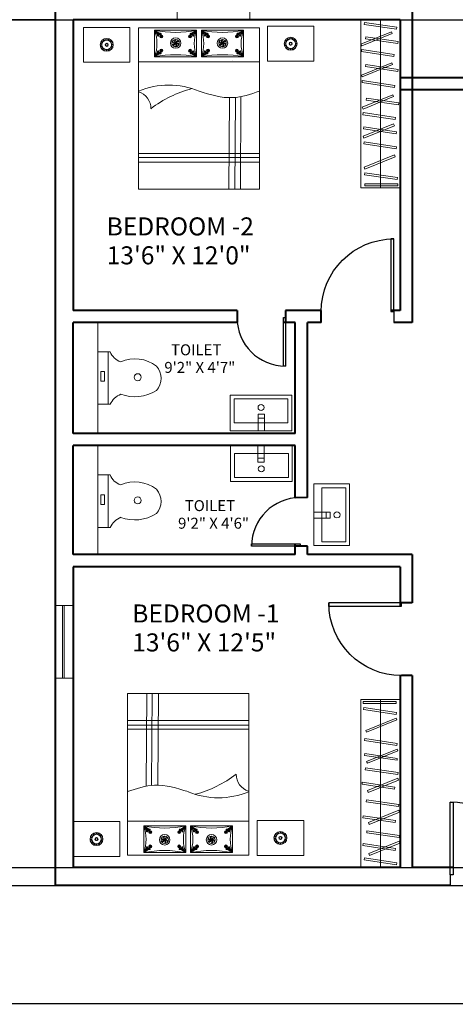
# Model space of a CAD drawing. Units: inches. Extents: x -46 to 1145, y -527 to 760.
# Tile 17 of 57: x 573 to 788, y -527 to -39. Entities that reach past the tile are written whole.
import ezdxf

# ---------------------------------------------------------------- set-up
doc = ezdxf.new("R2010")
doc.units = ezdxf.units.IN
doc.header["$MEASUREMENT"] = 0
for name, color, linetype, lineweight in [('A-ANNO-DIMS', 2, 'Continuous', 18), ('A-AREA-IDEN', 1, 'Continuous', 18), ('A-FLOR-CASE', 32, 'Continuous', 18), ('A-FLOR-FIXT', 9, 'Continuous', 18), ('A-FURN', 2, 'Continuous', 13), ('C-SITE', 7, 'Continuous', 30), ('DOORS', 3, 'Continuous', 25), ('WALLS', 4, 'Continuous', 40), ('WINDOWS', 240, 'Continuous', 20)]:
    doc.layers.add(name, color=color, linetype=linetype, lineweight=lineweight)
doc.layers.add('FURNTIURE', color=2, linetype='Continuous')
doc.layers.add('LT', color=9, linetype='Continuous')
doc.styles.get("Standard").update_dxf_attribs({"font": 'arial.ttf'})
doc.dimstyles.get("Standard").update_dxf_attribs({"dimtxt": 0.18, "dimasz": 0.18, "dimexe": 0.18, "dimexo": 0.0625, "dimgap": 0.09, "dimtad": 0, "dimtih": 1, "dimtoh": 1, "dimdec": 0, "dimzin": 0, "dimdsep": 46, "dimlunit": 3, "dimtxsty": 'Standard', "dimcen": 0.09, "dimadec": 0, "dimazin": 0, "dimtfac": 1, "dimtdec": 0, "dimtofl": 0, "dimtmove": 0, "dimatfit": 3, "dimfxl": 1, "dimtolj": 1, "dimtzin": 0, "dimarcsym": 0})

# ---------------------------------------------------------------- blocks, each defined once
blk = doc.blocks.new('*U2')
for p, q in [((0, 0), (0, -6)), ((40, 0), (40, -6))]:
    blk.add_line(p, q)
blk.add_lwpolyline([(0, 0), (0, 40), (1.75, 40), (1.75, 0)], close=True)
blk.add_arc((0, 0), 40, 0, 90)
blk = doc.blocks.new('*U89')
at = {"layer": 'FURNTIURE'}
blk.add_line((0, 0.42), (0, -0.42), dxfattribs=at)
blk = doc.blocks.new('*U90')
at = {"layer": 'FURNTIURE', "transparency": 16777216}
for p, rotation in [((590.11, 507), 36), ((590.89, 507.4), 17.99999999999997), ((592.61, 507.4), 341.9999999999999), ((593.39, 507), 324), ((588.97, 504.75), 90), ((589.1, 505.61), 72), ((589.1, 503.89), 108), ((589.5, 506.39), 54), ((589.5, 503.11), 126), ((590.11, 502.49), 144), ((590.89, 502.1), 162), ((592.61, 502.1), 197.9999999999999), ((593.39, 502.49), 216), ((594.01, 506.39), 306), ((594.01, 503.11), 234), ((594.4, 505.61), 288), ((594.4, 503.89), 252), ((594.54, 504.75), 270), ((591.75, 501.96), 180)]:
    blk.add_blockref('*U89', p, dxfattribs=dict(at, rotation=rotation))
blk.add_blockref('*U89', (591.75, 507.53), dxfattribs=at)
blk = doc.blocks.new('*U87')
at = {"layer": 'FURNTIURE'}
blk.add_line((0, 0.1), (0, -0.1), dxfattribs=at)
blk = doc.blocks.new('*U88')
at = {"layer": 'FURNTIURE', "transparency": 16777216}
for p, rotation in [((141.23, 121.04), 90), ((141.27, 121.25), 72), ((141.27, 120.83), 108), ((141.36, 121.43), 54), ((141.36, 120.65), 126), ((141.51, 121.58), 35.99999999999999), ((141.51, 120.5), 144), ((141.7, 121.67), 17.99999999999998), ((141.7, 120.4), 162), ((141.9, 120.37), 180), ((142.11, 121.67), 342), ((142.11, 120.4), 198), ((142.3, 121.58), 324), ((142.3, 120.5), 216), ((142.44, 121.43), 306), ((142.44, 120.65), 234), ((142.54, 121.25), 288), ((142.54, 120.83), 252), ((142.57, 121.04), 270)]:
    blk.add_blockref('*U87', p, dxfattribs=dict(at, rotation=rotation))
blk.add_blockref('*U87', (141.9, 121.71), dxfattribs=at)
blk = doc.blocks.new('NIGHTSTAND')
blk.add_lwpolyline([(23.06, 0), (0, 0), (0, 17.28), (23.06, 17.28)], close=True)
for radius in [3.21, 2.36, 0.77, 0.567]:
    blk.add_circle((11.53, 8.64), radius)
for name, p in [('*U90', (-580.22, -496.1)), ('*U88', (-130.37, -112.4))]:
    blk.add_blockref(name, p)
blk = doc.blocks.new('WARDROBE')
blk.add_line((9.78, 0), (9.78, 83.25))
for points in [[(19.56, 0), (0, 0), (0, 83.25), (19.56, 83.25)], [(17.74, 78.49), (1.66, 80.88), (1.8, 81.87), (17.88, 79.48)], [(15.55, 76.35), (0.49, 70.23), (0.11, 71.16), (15.17, 77.28)], [(18.43, 71.4), (2.35, 73.79), (2.5, 74.78), (18.58, 72.39)], [(16.47, 65.03), (0.39, 67.42), (0.54, 68.41), (16.62, 66.02)], [(15.79, 61), (0.73, 54.88), (0.35, 55.81), (15.41, 61.93)], [(18.43, 57.62), (2.35, 60.01), (2.5, 61), (18.58, 58.61)], [(16.71, 49.68), (0.63, 52.07), (0.78, 53.06), (16.86, 50.67)], [(16.22, 45.12), (1.16, 39), (0.78, 39.93), (15.84, 46.05)], [(18.77, 41.02), (2.69, 43.41), (2.84, 44.4), (18.92, 42.01)], [(17.14, 33.8), (1.06, 36.19), (1.21, 37.19), (17.29, 34.8)], [(16.65, 30.67), (1.59, 24.55), (1.21, 25.48), (16.27, 31.6)], [(17.52, 26.78), (1.44, 29.17), (1.59, 30.16), (17.67, 27.77)], [(17.57, 19.35), (1.49, 21.74), (1.64, 22.73), (17.72, 20.34)], [(17.08, 15.35), (2.02, 9.23), (1.64, 10.16), (16.7, 16.28)], [(18, 4.03), (1.92, 6.42), (2.07, 7.41), (18.15, 5.03)], [(18.32, 0.98), (2.07, 0.98), (2.07, 1.98), (18.32, 1.98)]]:
    blk.add_lwpolyline(points, close=True)
blk = doc.blocks.new('LAVATORY-RECT')
blk.add_line((14.01, 6.17), (17.08, 6.17))
for points in [[(30.61, 0), (0, 0), (0, 17.7), (30.61, 17.7)], [(28.7, 3.94), (1.97, 3.94), (1.97, 15.81), (28.7, 15.81)], [(17.08, 0), (14.01, 0), (14.01, 8.17), (17.08, 8.17)]]:
    blk.add_lwpolyline(points, close=True)
blk.add_circle((15.39, 11.51), 1.51)
blk = doc.blocks.new('WATER-CLOSET')
for p, q in [((0, 0), (0, 26.01)), ((0, 26.01), (6.13, 26.01)), ((5.22, 21.04), (5.22, 26.01)), ((5.22, 26.01), (5.22, 0)), ((0, 0), (6.13, 0))]:
    blk.add_line(p, q)
blk.add_lwpolyline([(1.51, 11.4), (1.51, 16.16), (3.34, 16.16), (3.34, 11.4)], close=True)
blk.add_circle((19.79, 13.37), 1.75)
for centre, radius, start, end in [((14.15, 29.2), 8.64, 201.6782, 251.0259), ((18.35, 4.96), 17.54, 52.4616, 113.5359), ((22.52, 12.84), 8.87, 317.2682, 42.7318), ((15.4, -4.5), 10.31, 113.1704, 154.0947), ((18.33, 23.71), 20, 249.5645, 302.3709)]:
    blk.add_arc(centre, radius, start, end)
blk = doc.blocks.new('WINDOW-36IN')
for p, q in [((0, 4.5), (0, 9)), ((0, 9), (0, 0)), ((0, 5.23), (36, 5.23)), ((36, 9), (36, 0)), ((0, 4.5), (36, 4.5))]:
    blk.add_line(p, q)
blk = doc.blocks.new('*U58')
at = {"layer": 'LT'}
blk.add_line((0, 0.28), (0, -0.28), dxfattribs=at)
for centre, start, end in [((0.73, 0), 159.0676, 200.9324), ((-0.73, 0), 339.0676, 20.9324)]:
    blk.add_arc(centre, 0.786, start, end, dxfattribs=at)
blk = doc.blocks.new('*U59')
at = {"layer": 'LT', "transparency": 16777216}
for p, rotation in [((609.66, 443.79), 80.00000000000001), ((609.76, 443.96), 40.00000000000002), ((610.12, 443.96), 320), ((610.21, 443.79), 280), ((609.69, 443.6), 120), ((609.84, 443.48), 160), ((610.03, 443.48), 200), ((610.18, 443.6), 240)]:
    blk.add_blockref('*U58', p, dxfattribs=dict(at, rotation=rotation))
blk.add_blockref('*U58', (609.94, 444.03), dxfattribs=at)
blk = doc.blocks.new('*U60')
at = {"layer": 'LT'}
blk.add_line((0, 0.12), (0, -0.12), dxfattribs=at)
for centre, start, end in [((0.31, 0), 159.0676, 200.9324), ((-0.31, 0), 339.0676, 20.9324)]:
    blk.add_arc(centre, 0.335, start, end, dxfattribs=at)
blk = doc.blocks.new('*U61')
at = {"layer": 'LT', "transparency": 16777216}
for p, rotation in [((259.5, 188.9), 80.00000000000001), ((259.51, 188.82), 120), ((259.54, 188.97), 40), ((259.57, 188.76), 160), ((259.65, 188.76), 200), ((259.69, 188.97), 320), ((259.72, 188.82), 240), ((259.73, 188.9), 280)]:
    blk.add_blockref('*U60', p, dxfattribs=dict(at, rotation=rotation))
blk.add_blockref('*U60', (259.61, 189), dxfattribs=at)
blk = doc.blocks.new('*U62')
at = {"layer": 'LT'}
blk.add_line((0, 0.12), (0, -0.12), dxfattribs=at)
for centre, start, end in [((0.31, 0), 159.0676, 200.9324), ((-0.31, 0), 339.0676, 20.9324)]:
    blk.add_arc(centre, 0.335, start, end, dxfattribs=at)
blk = doc.blocks.new('*U63')
at = {"layer": 'LT', "transparency": 16777216}
for p, rotation in [((259.5, 188.9), 80.00000000000001), ((259.51, 188.82), 120), ((259.54, 188.97), 40), ((259.57, 188.76), 160), ((259.65, 188.76), 200), ((259.69, 188.97), 320), ((259.72, 188.82), 240), ((259.73, 188.9), 280)]:
    blk.add_blockref('*U62', p, dxfattribs=dict(at, rotation=rotation))
blk.add_blockref('*U62', (259.61, 189), dxfattribs=at)
blk = doc.blocks.new('*U64')
at = {"layer": 'LT'}
blk.add_line((0, 0.28), (0, -0.28), dxfattribs=at)
for centre, start, end in [((0.73, 0), 159.0676, 200.9324), ((-0.73, 0), 339.0676, 20.9324)]:
    blk.add_arc(centre, 0.786, start, end, dxfattribs=at)
blk = doc.blocks.new('*U65')
at = {"layer": 'LT', "transparency": 16777216}
for p, rotation in [((609.66, 443.79), 80.00000000000001), ((609.76, 443.96), 40.00000000000002), ((610.12, 443.96), 320), ((610.21, 443.79), 280), ((609.69, 443.6), 120), ((609.84, 443.48), 160), ((610.03, 443.48), 200), ((610.18, 443.6), 240)]:
    blk.add_blockref('*U64', p, dxfattribs=dict(at, rotation=rotation))
blk.add_blockref('*U64', (609.94, 444.03), dxfattribs=at)
blk = doc.blocks.new('*U66')
at = {"layer": 'LT'}
blk.add_line((0, 0.12), (0, -0.12), dxfattribs=at)
for centre, start, end in [((0.31, 0), 159.0676, 200.9324), ((-0.31, 0), 339.0676, 20.9324)]:
    blk.add_arc(centre, 0.335, start, end, dxfattribs=at)
blk = doc.blocks.new('*U67')
at = {"layer": 'LT', "transparency": 16777216}
for p, rotation in [((259.5, 188.9), 80.00000000000001), ((259.51, 188.82), 120), ((259.54, 188.97), 40), ((259.57, 188.76), 160), ((259.65, 188.76), 200), ((259.69, 188.97), 320), ((259.72, 188.82), 240), ((259.73, 188.9), 280)]:
    blk.add_blockref('*U66', p, dxfattribs=dict(at, rotation=rotation))
blk.add_blockref('*U66', (259.61, 189), dxfattribs=at)
blk = doc.blocks.new('*U68')
at = {"layer": 'LT'}
blk.add_line((0, 0.12), (0, -0.12), dxfattribs=at)
for centre, start, end in [((0.31, 0), 159.0676, 200.9324), ((-0.31, 0), 339.0676, 20.9324)]:
    blk.add_arc(centre, 0.335, start, end, dxfattribs=at)
blk = doc.blocks.new('*U69')
at = {"layer": 'LT', "transparency": 16777216}
for p, rotation in [((259.5, 188.9), 80.00000000000001), ((259.51, 188.82), 120), ((259.54, 188.97), 40), ((259.57, 188.76), 160), ((259.65, 188.76), 200), ((259.69, 188.97), 320), ((259.72, 188.82), 240), ((259.73, 188.9), 280)]:
    blk.add_blockref('*U68', p, dxfattribs=dict(at, rotation=rotation))
blk.add_blockref('*U68', (259.61, 189), dxfattribs=at)
blk = doc.blocks.new('*U70')
at = {"layer": 'LT'}
blk.add_line((0, 0.28), (0, -0.28), dxfattribs=at)
for centre, start, end in [((0.73, 0), 159.0676, 200.9324), ((-0.73, 0), 339.0676, 20.9324)]:
    blk.add_arc(centre, 0.786, start, end, dxfattribs=at)
blk = doc.blocks.new('*U71')
at = {"layer": 'LT', "transparency": 16777216}
for p, rotation in [((609.66, 443.79), 80.00000000000001), ((609.76, 443.96), 40.00000000000002), ((610.12, 443.96), 320), ((610.21, 443.79), 280), ((609.69, 443.6), 120), ((609.84, 443.48), 160), ((610.03, 443.48), 200), ((610.18, 443.6), 240)]:
    blk.add_blockref('*U70', p, dxfattribs=dict(at, rotation=rotation))
blk.add_blockref('*U70', (609.94, 444.03), dxfattribs=at)
blk = doc.blocks.new('*U46')
at = {"layer": 'LT'}
blk.add_line((0, 0.12), (0, -0.12), dxfattribs=at)
for centre, start, end in [((0.31, 0), 159.0676, 200.9324), ((-0.31, 0), 339.0676, 20.9324)]:
    blk.add_arc(centre, 0.335, start, end, dxfattribs=at)
blk = doc.blocks.new('*U47')
at = {"layer": 'LT', "transparency": 16777216}
for p, rotation in [((259.5, 188.9), 80.00000000000001), ((259.51, 188.82), 120), ((259.54, 188.97), 40), ((259.57, 188.76), 160), ((259.65, 188.76), 200), ((259.69, 188.97), 320), ((259.72, 188.82), 240), ((259.73, 188.9), 280)]:
    blk.add_blockref('*U46', p, dxfattribs=dict(at, rotation=rotation))
blk.add_blockref('*U46', (259.61, 189), dxfattribs=at)
blk = doc.blocks.new('*U48')
at = {"layer": 'LT'}
blk.add_line((0, 0.12), (0, -0.12), dxfattribs=at)
for centre, start, end in [((0.31, 0), 159.0676, 200.9324), ((-0.31, 0), 339.0676, 20.9324)]:
    blk.add_arc(centre, 0.335, start, end, dxfattribs=at)
blk = doc.blocks.new('*U49')
at = {"layer": 'LT', "transparency": 16777216}
for p, rotation in [((259.5, 188.9), 80.00000000000001), ((259.51, 188.82), 120), ((259.54, 188.97), 40), ((259.57, 188.76), 160), ((259.65, 188.76), 200), ((259.69, 188.97), 320), ((259.72, 188.82), 240), ((259.73, 188.9), 280)]:
    blk.add_blockref('*U48', p, dxfattribs=dict(at, rotation=rotation))
blk.add_blockref('*U48', (259.61, 189), dxfattribs=at)
blk = doc.blocks.new('*U50')
at = {"layer": 'LT'}
blk.add_line((0, 0.28), (0, -0.28), dxfattribs=at)
for centre, start, end in [((0.73, 0), 159.0676, 200.9324), ((-0.73, 0), 339.0676, 20.9324)]:
    blk.add_arc(centre, 0.786, start, end, dxfattribs=at)
blk = doc.blocks.new('*U51')
at = {"layer": 'LT', "transparency": 16777216}
for p, rotation in [((609.66, 443.79), 80.00000000000001), ((609.76, 443.96), 40.00000000000002), ((610.12, 443.96), 320), ((610.21, 443.79), 280), ((609.69, 443.6), 120), ((609.84, 443.48), 160), ((610.03, 443.48), 200), ((610.18, 443.6), 240)]:
    blk.add_blockref('*U50', p, dxfattribs=dict(at, rotation=rotation))
blk.add_blockref('*U50', (609.94, 444.03), dxfattribs=at)
blk = doc.blocks.new('*U52')
at = {"layer": 'LT'}
blk.add_line((0, 0.12), (0, -0.12), dxfattribs=at)
for centre, start, end in [((0.31, 0), 159.0676, 200.9324), ((-0.31, 0), 339.0676, 20.9324)]:
    blk.add_arc(centre, 0.335, start, end, dxfattribs=at)
blk = doc.blocks.new('*U53')
at = {"layer": 'LT', "transparency": 16777216}
for p, rotation in [((259.5, 188.9), 80.00000000000001), ((259.51, 188.82), 120), ((259.54, 188.97), 40), ((259.57, 188.76), 160), ((259.65, 188.76), 200), ((259.69, 188.97), 320), ((259.72, 188.82), 240), ((259.73, 188.9), 280)]:
    blk.add_blockref('*U52', p, dxfattribs=dict(at, rotation=rotation))
blk.add_blockref('*U52', (259.61, 189), dxfattribs=at)
blk = doc.blocks.new('*U54')
at = {"layer": 'LT'}
blk.add_line((0, 0.12), (0, -0.12), dxfattribs=at)
for centre, start, end in [((0.31, 0), 159.0676, 200.9324), ((-0.31, 0), 339.0676, 20.9324)]:
    blk.add_arc(centre, 0.335, start, end, dxfattribs=at)
blk = doc.blocks.new('*U55')
at = {"layer": 'LT', "transparency": 16777216}
for p, rotation in [((259.5, 188.9), 80.00000000000001), ((259.51, 188.82), 120), ((259.54, 188.97), 40), ((259.57, 188.76), 160), ((259.65, 188.76), 200), ((259.69, 188.97), 320), ((259.72, 188.82), 240), ((259.73, 188.9), 280)]:
    blk.add_blockref('*U54', p, dxfattribs=dict(at, rotation=rotation))
blk.add_blockref('*U54', (259.61, 189), dxfattribs=at)
blk = doc.blocks.new('*U34')
at = {"layer": 'LT'}
blk.add_line((0, 0.28), (0, -0.28), dxfattribs=at)
for centre, start, end in [((0.73, 0), 159.0676, 200.9324), ((-0.73, 0), 339.0676, 20.9324)]:
    blk.add_arc(centre, 0.786, start, end, dxfattribs=at)
blk = doc.blocks.new('*U35')
at = {"layer": 'LT', "transparency": 16777216}
for p, rotation in [((609.66, 443.79), 80.00000000000001), ((609.76, 443.96), 40.00000000000002), ((610.12, 443.96), 320), ((610.21, 443.79), 280), ((609.69, 443.6), 120), ((609.84, 443.48), 160), ((610.03, 443.48), 200), ((610.18, 443.6), 240)]:
    blk.add_blockref('*U34', p, dxfattribs=dict(at, rotation=rotation))
blk.add_blockref('*U34', (609.94, 444.03), dxfattribs=at)
blk = doc.blocks.new('*U36')
at = {"layer": 'LT'}
blk.add_line((0, 0.12), (0, -0.12), dxfattribs=at)
for centre, start, end in [((0.31, 0), 159.0676, 200.9324), ((-0.31, 0), 339.0676, 20.9324)]:
    blk.add_arc(centre, 0.335, start, end, dxfattribs=at)
blk = doc.blocks.new('*U37')
at = {"layer": 'LT', "transparency": 16777216}
for p, rotation in [((259.5, 188.9), 80.00000000000001), ((259.51, 188.82), 120), ((259.54, 188.97), 40), ((259.57, 188.76), 160), ((259.65, 188.76), 200), ((259.69, 188.97), 320), ((259.72, 188.82), 240), ((259.73, 188.9), 280)]:
    blk.add_blockref('*U36', p, dxfattribs=dict(at, rotation=rotation))
blk.add_blockref('*U36', (259.61, 189), dxfattribs=at)
blk = doc.blocks.new('*U38')
at = {"layer": 'LT'}
blk.add_line((0, 0.12), (0, -0.12), dxfattribs=at)
for centre, start, end in [((0.31, 0), 159.0676, 200.9324), ((-0.31, 0), 339.0676, 20.9324)]:
    blk.add_arc(centre, 0.335, start, end, dxfattribs=at)
blk = doc.blocks.new('*U39')
at = {"layer": 'LT', "transparency": 16777216}
for p, rotation in [((259.5, 188.9), 80.00000000000001), ((259.51, 188.82), 120), ((259.54, 188.97), 40), ((259.57, 188.76), 160), ((259.65, 188.76), 200), ((259.69, 188.97), 320), ((259.72, 188.82), 240), ((259.73, 188.9), 280)]:
    blk.add_blockref('*U38', p, dxfattribs=dict(at, rotation=rotation))
blk.add_blockref('*U38', (259.61, 189), dxfattribs=at)
blk = doc.blocks.new('*U40')
at = {"layer": 'LT'}
blk.add_line((0, 0.28), (0, -0.28), dxfattribs=at)
for centre, start, end in [((0.73, 0), 159.0676, 200.9324), ((-0.73, 0), 339.0676, 20.9324)]:
    blk.add_arc(centre, 0.786, start, end, dxfattribs=at)
blk = doc.blocks.new('*U41')
at = {"layer": 'LT', "transparency": 16777216}
for p, rotation in [((609.66, 443.79), 80.00000000000001), ((609.76, 443.96), 40.00000000000002), ((610.12, 443.96), 320), ((610.21, 443.79), 280), ((609.69, 443.6), 120), ((609.84, 443.48), 160), ((610.03, 443.48), 200), ((610.18, 443.6), 240)]:
    blk.add_blockref('*U40', p, dxfattribs=dict(at, rotation=rotation))
blk.add_blockref('*U40', (609.94, 444.03), dxfattribs=at)
blk = doc.blocks.new('*U42')
at = {"layer": 'LT'}
blk.add_line((0, 0.12), (0, -0.12), dxfattribs=at)
for centre, start, end in [((0.31, 0), 159.0676, 200.9324), ((-0.31, 0), 339.0676, 20.9324)]:
    blk.add_arc(centre, 0.335, start, end, dxfattribs=at)
blk = doc.blocks.new('*U43')
at = {"layer": 'LT', "transparency": 16777216}
for p, rotation in [((259.5, 188.9), 80.00000000000001), ((259.51, 188.82), 120), ((259.54, 188.97), 40), ((259.57, 188.76), 160), ((259.65, 188.76), 200), ((259.69, 188.97), 320), ((259.72, 188.82), 240), ((259.73, 188.9), 280)]:
    blk.add_blockref('*U42', p, dxfattribs=dict(at, rotation=rotation))
blk.add_blockref('*U42', (259.61, 189), dxfattribs=at)
blk = doc.blocks.new('*U44')
at = {"layer": 'LT'}
blk.add_line((0, 0.12), (0, -0.12), dxfattribs=at)
for centre, start, end in [((0.31, 0), 159.0676, 200.9324), ((-0.31, 0), 339.0676, 20.9324)]:
    blk.add_arc(centre, 0.335, start, end, dxfattribs=at)
blk = doc.blocks.new('*U45')
at = {"layer": 'LT', "transparency": 16777216}
for p, rotation in [((259.5, 188.9), 80.00000000000001), ((259.51, 188.82), 120), ((259.54, 188.97), 40), ((259.57, 188.76), 160), ((259.65, 188.76), 200), ((259.69, 188.97), 320), ((259.72, 188.82), 240), ((259.73, 188.9), 280)]:
    blk.add_blockref('*U44', p, dxfattribs=dict(at, rotation=rotation))
blk.add_blockref('*U44', (259.61, 189), dxfattribs=at)
blk = doc.blocks.new('*U72')
at = {"layer": 'LT'}
blk.add_line((0, 0.28), (0, -0.28), dxfattribs=at)
for centre, start, end in [((0.73, 0), 159.0676, 200.9324), ((-0.73, 0), 339.0676, 20.9324)]:
    blk.add_arc(centre, 0.786, start, end, dxfattribs=at)
blk = doc.blocks.new('*U73')
at = {"layer": 'LT', "transparency": 16777216}
for p, rotation in [((609.66, 443.79), 80.00000000000001), ((609.76, 443.96), 40.00000000000002), ((610.12, 443.96), 320), ((610.21, 443.79), 280), ((609.69, 443.6), 120), ((609.84, 443.48), 160), ((610.03, 443.48), 200), ((610.18, 443.6), 240)]:
    blk.add_blockref('*U72', p, dxfattribs=dict(at, rotation=rotation))
blk.add_blockref('*U72', (609.94, 444.03), dxfattribs=at)
blk = doc.blocks.new('*U74')
at = {"layer": 'LT'}
blk.add_line((0, 0.12), (0, -0.12), dxfattribs=at)
for centre, start, end in [((0.31, 0), 159.0676, 200.9324), ((-0.31, 0), 339.0676, 20.9324)]:
    blk.add_arc(centre, 0.335, start, end, dxfattribs=at)
blk = doc.blocks.new('*U75')
at = {"layer": 'LT', "transparency": 16777216}
for p, rotation in [((259.5, 188.9), 80.00000000000001), ((259.51, 188.82), 120), ((259.54, 188.97), 40), ((259.57, 188.76), 160), ((259.65, 188.76), 200), ((259.69, 188.97), 320), ((259.72, 188.82), 240), ((259.73, 188.9), 280)]:
    blk.add_blockref('*U74', p, dxfattribs=dict(at, rotation=rotation))
blk.add_blockref('*U74', (259.61, 189), dxfattribs=at)
blk = doc.blocks.new('*U76')
at = {"layer": 'LT'}
blk.add_line((0, 0.12), (0, -0.12), dxfattribs=at)
for centre, start, end in [((0.31, 0), 159.0676, 200.9324), ((-0.31, 0), 339.0676, 20.9324)]:
    blk.add_arc(centre, 0.335, start, end, dxfattribs=at)
blk = doc.blocks.new('*U77')
at = {"layer": 'LT', "transparency": 16777216}
for p, rotation in [((259.5, 188.9), 80.00000000000001), ((259.51, 188.82), 120), ((259.54, 188.97), 40), ((259.57, 188.76), 160), ((259.65, 188.76), 200), ((259.69, 188.97), 320), ((259.72, 188.82), 240), ((259.73, 188.9), 280)]:
    blk.add_blockref('*U76', p, dxfattribs=dict(at, rotation=rotation))
blk.add_blockref('*U76', (259.61, 189), dxfattribs=at)
blk = doc.blocks.new('*U78')
at = {"layer": 'LT'}
blk.add_line((0, 0.28), (0, -0.28), dxfattribs=at)
for centre, start, end in [((0.73, 0), 159.0676, 200.9324), ((-0.73, 0), 339.0676, 20.9324)]:
    blk.add_arc(centre, 0.786, start, end, dxfattribs=at)
blk = doc.blocks.new('*U79')
at = {"layer": 'LT', "transparency": 16777216}
for p, rotation in [((609.66, 443.79), 80.00000000000001), ((609.76, 443.96), 40.00000000000002), ((610.12, 443.96), 320), ((610.21, 443.79), 280), ((609.69, 443.6), 120), ((609.84, 443.48), 160), ((610.03, 443.48), 200), ((610.18, 443.6), 240)]:
    blk.add_blockref('*U78', p, dxfattribs=dict(at, rotation=rotation))
blk.add_blockref('*U78', (609.94, 444.03), dxfattribs=at)
blk = doc.blocks.new('*U80')
at = {"layer": 'LT'}
blk.add_line((0, 0.12), (0, -0.12), dxfattribs=at)
for centre, start, end in [((0.31, 0), 159.0676, 200.9324), ((-0.31, 0), 339.0676, 20.9324)]:
    blk.add_arc(centre, 0.335, start, end, dxfattribs=at)
blk = doc.blocks.new('*U81')
at = {"layer": 'LT', "transparency": 16777216}
for p, rotation in [((259.5, 188.9), 80.00000000000001), ((259.51, 188.82), 120), ((259.54, 188.97), 40), ((259.57, 188.76), 160), ((259.65, 188.76), 200), ((259.69, 188.97), 320), ((259.72, 188.82), 240), ((259.73, 188.9), 280)]:
    blk.add_blockref('*U80', p, dxfattribs=dict(at, rotation=rotation))
blk.add_blockref('*U80', (259.61, 189), dxfattribs=at)
blk = doc.blocks.new('*U82')
at = {"layer": 'LT'}
blk.add_line((0, 0.12), (0, -0.12), dxfattribs=at)
for centre, start, end in [((0.31, 0), 159.0676, 200.9324), ((-0.31, 0), 339.0676, 20.9324)]:
    blk.add_arc(centre, 0.335, start, end, dxfattribs=at)
blk = doc.blocks.new('*U83')
at = {"layer": 'LT', "transparency": 16777216}
for p, rotation in [((259.5, 188.9), 80.00000000000001), ((259.51, 188.82), 120), ((259.54, 188.97), 40), ((259.57, 188.76), 160), ((259.65, 188.76), 200), ((259.69, 188.97), 320), ((259.72, 188.82), 240), ((259.73, 188.9), 280)]:
    blk.add_blockref('*U82', p, dxfattribs=dict(at, rotation=rotation))
blk.add_blockref('*U82', (259.61, 189), dxfattribs=at)
blk = doc.blocks.new('*U32')
at = {"layer": 'FURNTIURE'}
blk.add_open_spline([(0.04, 1.82), (-0.22, 1.45), (-0.66, 0.8), (0.1, -0.02), (0.64, -0.93), (0.24, -1.53), (0.04, -1.82)], degree=3, knots=[0, 0, 0, 0, 1.177175, 2.037162, 3.056205, 4.032246, 4.032246, 4.032246, 4.032246], dxfattribs=at)
blk = doc.blocks.new('*U33')
at = {"layer": 'FURNTIURE', "transparency": 16777216}
for p, rotation in [((904.32, 663.42), 300), ((904.32, 663.35), 59.99999999999999), ((904.36, 663.42), 239.9999999999999), ((904.36, 663.35), 119.9999999999999), ((904.38, 663.38), 180)]:
    blk.add_blockref('*U32', p, dxfattribs=dict(at, rotation=rotation))
blk.add_blockref('*U32', (904.3, 663.38), dxfattribs=at)
blk = doc.blocks.new('*U56')
at = {"layer": 'FURNTIURE'}
blk.add_open_spline([(0.04, 1.82), (-0.22, 1.45), (-0.66, 0.8), (0.1, -0.02), (0.64, -0.93), (0.24, -1.53), (0.04, -1.82)], degree=3, knots=[0, 0, 0, 0, 1.177175, 2.037162, 3.056205, 4.032246, 4.032246, 4.032246, 4.032246], dxfattribs=at)
blk = doc.blocks.new('*U57')
at = {"layer": 'FURNTIURE', "transparency": 16777216}
for p, rotation in [((904.32, 663.42), 300), ((904.32, 663.35), 59.99999999999999), ((904.36, 663.42), 239.9999999999999), ((904.36, 663.35), 119.9999999999999), ((904.38, 663.38), 180)]:
    blk.add_blockref('*U56', p, dxfattribs=dict(at, rotation=rotation))
blk.add_blockref('*U56', (904.3, 663.38), dxfattribs=at)
blk = doc.blocks.new('BED-QUEEN-FURNISHED')
for p, q in [((0, 0), (0, 80)), ((0, 80), (60, 80)), ((8, 78.8), (28.8, 78.8)), ((8, 65.6), (8, 78.8)), ((8, 78.8), (11.38, 75.61)), ((8, 78.8), (9.68, 76.18)), ((8, 78.8), (10.93, 76.98)), ((28.8, 78.8), (25.41, 75.61)), ((28.8, 78.8), (25.87, 76.98)), ((28.8, 78.8), (27.12, 76.18)), ((28.8, 78.8), (28.8, 65.6)), ((31.2, 78.8), (52, 78.8)), ((31.2, 65.6), (31.2, 78.8)), ((31.2, 78.8), (52, 78.8)), ((31.2, 65.6), (31.2, 78.8)), ((31.2, 78.8), (34.58, 75.61)), ((31.2, 78.8), (32.88, 76.18)), ((31.2, 78.8), (34.13, 76.98)), ((52, 78.8), (48.61, 75.61)), ((52, 78.8), (49.07, 76.98)), ((52, 78.8), (50.32, 76.18)), ((52, 78.8), (52, 65.6)), ((52, 78.8), (52, 65.6)), ((60, 80), (60, 0)), ((10.93, 76.98), (10.93, 76.75)), ((11.25, 75.74), (11.25, 75.18)), ((25.55, 75.74), (25.55, 75.18)), ((25.87, 76.98), (25.87, 76.75)), ((27.12, 76.18), (27.12, 75.95)), ((34.13, 76.98), (34.13, 76.75)), ((34.45, 75.74), (34.45, 75.18)), ((48.75, 75.74), (48.75, 75.18)), ((49.07, 76.98), (49.07, 76.75)), ((50.32, 76.18), (50.32, 75.95)), ((8, 65.61), (11.38, 68.8)), ((11.25, 68.67), (11.25, 69.23)), ((28.8, 65.6), (25.41, 68.79)), ((27.11, 68.22), (27.11, 68.46)), ((31.2, 65.61), (34.58, 68.8)), ((34.45, 68.67), (34.45, 69.23)), ((52, 65.6), (48.61, 68.79)), ((50.31, 68.22), (50.31, 68.46)), ((8, 65.61), (9.68, 68.23)), ((8, 65.61), (10.92, 67.43)), ((8, 65.6), (28.8, 65.6)), ((10.92, 67.43), (10.92, 67.67)), ((25.87, 67.42), (25.87, 67.66)), ((28.8, 65.6), (25.87, 67.42)), ((28.8, 65.6), (27.11, 68.22)), ((31.2, 65.61), (32.88, 68.23)), ((31.2, 65.61), (34.12, 67.43)), ((31.2, 65.6), (52, 65.6)), ((31.2, 65.6), (52, 65.6)), ((34.12, 67.43), (34.12, 67.67)), ((46.8, 63.6), (46.8, 63.6)), ((49.07, 67.42), (49.07, 67.66)), ((52, 65.6), (49.07, 67.42)), ((52, 65.6), (50.31, 68.22)), ((60, 63.2), (0, 63.2)), ((44.72, 0), (45.02, 45.37)), ((47.8, 0), (48.1, 45.5)), ((50.46, 0), (50.76, 45.91)), ((0, 17.7), (60, 17.7)), ((0, 15.69), (60, 15.69)), ((0, 13.42), (60, 13.42)), ((60, 0), (0, 0))]:
    blk.add_line(p, q)
for centre, radius in [((9.68, 76.18), 0.308), ((9.68, 76.18), 0.239), ((11.25, 75.74), 0.723), ((10.93, 76.98), 0.308), ((10.93, 76.98), 0.239), ((11.25, 75.74), 0.562), ((18.4, 72.44), 2.6), ((18.4, 72.44), 1.82), ((25.55, 75.74), 0.723), ((25.55, 75.74), 0.562), ((25.87, 76.98), 0.308), ((25.87, 76.98), 0.239), ((27.12, 76.18), 0.308), ((27.12, 76.18), 0.239), ((32.88, 76.18), 0.308), ((32.88, 76.18), 0.239), ((34.45, 75.74), 0.723), ((34.13, 76.98), 0.308), ((34.13, 76.98), 0.239), ((34.45, 75.74), 0.562), ((41.6, 72.44), 2.6), ((41.6, 72.44), 1.82), ((48.75, 75.74), 0.723), ((48.75, 75.74), 0.562), ((49.07, 76.98), 0.308), ((49.07, 76.98), 0.239), ((50.32, 76.18), 0.308), ((50.32, 76.18), 0.239), ((9.68, 68.23), 0.308), ((9.68, 68.23), 0.239), ((11.25, 68.67), 0.723), ((11.25, 68.67), 0.562), ((25.55, 68.66), 0.723), ((25.55, 68.66), 0.562), ((27.11, 68.22), 0.308), ((27.11, 68.22), 0.239), ((32.88, 68.23), 0.308), ((32.88, 68.23), 0.239), ((34.45, 68.67), 0.723), ((34.45, 68.67), 0.562), ((48.75, 68.66), 0.723), ((48.75, 68.66), 0.562), ((50.31, 68.22), 0.308), ((50.31, 68.22), 0.239), ((10.92, 67.43), 0.308), ((10.92, 67.43), 0.239), ((25.87, 67.42), 0.308), ((25.87, 67.42), 0.239), ((34.12, 67.43), 0.308), ((34.12, 67.43), 0.239), ((49.07, 67.42), 0.308), ((49.07, 67.42), 0.239)]:
    blk.add_circle(centre, radius)
for centre, radius, start, end in [((18.4, 129.18), 51.44, 258.3356, 281.6644), ((-10.65, 72.2), 19.79, 340.5151, 19.4849), ((47.45, 72.2), 19.79, 160.5151, 199.4849), ((41.6, 129.18), 51.44, 258.3356, 281.6644), ((12.55, 72.2), 19.79, 340.5151, 19.4849), ((70.65, 72.2), 19.79, 160.5151, 199.4849), ((11.24, 76.86), 0.335, 159.0676, 200.9324), ((10.61, 76.86), 0.335, 339.0676, 20.9324), ((11.99, 75.46), 0.786, 159.0676, 200.9324), ((10.52, 75.46), 0.786, 339.0676, 20.9324), ((26.28, 75.46), 0.786, 159.0676, 200.9324), ((24.81, 75.46), 0.786, 339.0676, 20.9324), ((26.19, 76.86), 0.335, 159.0676, 200.9324), ((25.56, 76.86), 0.335, 339.0676, 20.9324), ((27.43, 76.06), 0.335, 159.0676, 200.9324), ((26.8, 76.06), 0.335, 339.0676, 20.9324), ((34.44, 76.86), 0.335, 159.0676, 200.9324), ((33.81, 76.86), 0.335, 339.0676, 20.9324), ((35.19, 75.46), 0.786, 159.0676, 200.9324), ((33.72, 75.46), 0.786, 339.0676, 20.9324), ((49.48, 75.46), 0.786, 159.0676, 200.9324), ((48.01, 75.46), 0.786, 339.0676, 20.9324), ((49.39, 76.86), 0.335, 159.0676, 200.9324), ((48.76, 76.86), 0.335, 339.0676, 20.9324), ((50.63, 76.06), 0.335, 159.0676, 200.9324), ((50, 76.06), 0.335, 339.0676, 20.9324), ((11.98, 68.95), 0.786, 159.028, 200.8928), ((10.51, 68.95), 0.786, 339.028, 20.8928), ((27.43, 68.34), 0.335, 159.028, 200.8928), ((26.8, 68.34), 0.335, 339.028, 20.8928), ((35.18, 68.95), 0.786, 159.028, 200.8928), ((33.71, 68.95), 0.786, 339.028, 20.8928), ((50.63, 68.34), 0.335, 159.028, 200.8928), ((50, 68.34), 0.335, 339.028, 20.8928), ((18.4, 15.22), 51.44, 78.3356, 101.6644), ((11.24, 67.55), 0.335, 159.028, 200.8928), ((10.61, 67.55), 0.335, 339.028, 20.8928), ((26.18, 67.54), 0.335, 159.028, 200.8928), ((25.56, 67.54), 0.335, 339.028, 20.8928), ((41.6, 15.22), 51.44, 78.3356, 101.6644), ((34.44, 67.55), 0.335, 159.028, 200.8928), ((33.81, 67.55), 0.335, 339.028, 20.8928), ((49.38, 67.54), 0.335, 159.028, 200.8928), ((48.76, 67.54), 0.335, 339.028, 20.8928), ((15, 13.08), 38.56, 67.1089, 112.8911), ((40.88, -5.13), 56.88, 104.6834, 127.6009), ((-2.62, 39.94), 8.8, 0, 72.6522), ((40.88, -5.13), 56.88, 70.3635, 70.606)]:
    blk.add_arc(centre, radius, start, end)
blk.add_open_spline([(30, 48.6), (35.57, 46.87), (45.64, 43.74), (55.56, 47.1), (60, 48.6)], degree=3, knots=[0, 0, 0, 0, 16.971495, 30.687365, 30.687365, 30.687365, 30.687365])
at = {"xscale": -1}
for name, p in [('*U43', (269.3, -112.69)), ('*U45', (270.54, -111.89)), ('*U41', (621.19, -368.01)), ('*U67', (292.5, -112.69)), ('*U69', (293.74, -111.89)), ('*U65', (644.39, -368.01))]:
    blk.add_blockref(name, p, dxfattribs=at)
for name, p in [('*U33', (-885.94, -590.95)), ('*U35', (-584.39, -368.01)), ('*U39', (-233.74, -111.89)), ('*U37', (-232.5, -112.69)), ('*U57', (-862.74, -590.95)), ('*U59', (-561.19, -368.01)), ('*U63', (-210.54, -111.89)), ('*U61', (-209.3, -112.69))]:
    blk.add_blockref(name, p)
at = {"rotation": 179.9603994254766}
for name, p in [('*U81', (269.43, 256.92)), ('*U79', (621.49, 512)), ('*U53', (292.63, 256.92)), ('*U51', (644.69, 512)), ('*U83', (270.67, 256.12)), ('*U55', (293.87, 256.12))]:
    blk.add_blockref(name, p, dxfattribs=at)
at = {"xscale": -1, "rotation": 179.9603994254766}
for name, p in [('*U73', (-584.08, 512.83)), ('*U75', (-232.37, 257.27)), ('*U71', (-560.88, 512.83)), ('*U47', (-209.17, 257.27)), ('*U77', (-233.61, 256.47)), ('*U49', (-210.41, 256.47))]:
    blk.add_blockref(name, p, dxfattribs=at)
blk = doc.blocks.new('*D684')
at = {"layer": 'A-ANNO-DIMS', "color": 0, "lineweight": -2, "transparency": 16777216}
for p, q in [((12.56, -468.54), (12.56, -527.26)), ((1086.56, -468.54), (1086.56, -527.26)), ((12.74, -527.08), (549.21, -527.08)), ((1086.38, -527.08), (549.91, -527.08))]:
    blk.add_line(p, q, dxfattribs=at)
at = {"layer": 'A-ANNO-DIMS', "color": 0, "transparency": 16777216}
for points in [[(12.74, -527.05), (12.74, -527.11), (12.56, -527.08)], [(1086.38, -527.05), (1086.38, -527.11), (1086.56, -527.08)]]:
    blk.add_solid(points, dxfattribs=at)
at = {"layer": 'Defpoints', "color": 0, "transparency": 16777216}
for p in [(12.56, -468.48), (1086.56, -468.48), (1086.56, -527.08)]:
    blk.add_point(p, dxfattribs=at)
at = {"layer": 'A-ANNO-DIMS', "color": 0, "transparency": 16777216, "insert": (549.56, -527.08), "char_height": 0.18, "attachment_point": 5}
blk.add_mtext('\\A1;1074', dxfattribs=at)
blk = doc.blocks.new('*D702')
at = {"layer": 'A-ANNO-DIMS', "color": 0, "lineweight": -2, "transparency": 16777216}
for p, q in [((189.63, -39.48), (1145.34, -39.48)), ((1145.16, -39.66), (1145.16, -249.3)), ((1145.16, -459.3), (1145.16, -249.66)), ((183.63, -459.48), (1145.34, -459.48))]:
    blk.add_line(p, q, dxfattribs=at)
at = {"layer": 'A-ANNO-DIMS', "color": 0, "transparency": 16777216}
for points in [[(1145.13, -39.66), (1145.19, -39.66), (1145.16, -39.48)], [(1145.13, -459.3), (1145.19, -459.3), (1145.16, -459.48)]]:
    blk.add_solid(points, dxfattribs=at)
at = {"layer": 'Defpoints', "color": 0, "transparency": 16777216}
for p in [(189.56, -39.48), (1145.16, -39.48), (183.56, -459.48)]:
    blk.add_point(p, dxfattribs=at)
at = {"layer": 'A-ANNO-DIMS', "color": 0, "transparency": 16777216, "insert": (1145.16, -249.48), "char_height": 0.18, "attachment_point": 5}
blk.add_mtext('\\A1;420', dxfattribs=at)

msp = doc.modelspace()

# ---------------------------------------------------------------- linework, layer by layer
at = {"layer": 'A-FLOR-CASE'}
for p, q in [((611.2427, -189.4824), (611.2427, -244.4824)), ((611.2427, -250.4824), (611.2427, -304.4824))]:
    msp.add_line(p, q, dxfattribs=at)
at = {"layer": 'C-SITE'}
for p, q in [((590.0637, -39.4824), (189.5637, -39.4824)), ((21.5637, -459.4824), (1077.5637, -459.4824)), ((12.5637, -468.4824), (1086.5637, -468.4824))]:
    msp.add_line(p, q, dxfattribs=at)
at = {"layer": 'WALLS'}
for p, q in [((590.0637, -30.4824), (590.0637, -468.4824)), ((767.0637, -30.4824), (767.0637, -189.4824)), ((599.0637, -39.4824), (599.0637, -183.4824)), ((761.0637, -39.4824), (599.0637, -39.4824)), ((761.0637, -39.4824), (761.0637, -183.4824)), ((761.0637, -68.1114), (911.0637, -68.1114)), ((761.0637, -74.1114), (911.0637, -74.1114)), ((680.2169, -183.4824), (599.0637, -183.4824)), ((680.2169, -183.4824), (680.3372, -189.4824)), ((721.9431, -183.4824), (704.2169, -183.4824)), ((704.2169, -183.4824), (704.2169, -189.4824)), ((721.9381, -189.4824), (721.9381, -183.4824)), ((761.0637, -183.4824), (756.3631, -183.4824)), ((757.9381, -184.0824), (757.9381, -183.4824)), ((680.3372, -189.4824), (599.0637, -189.4824)), ((599.0637, -244.4824), (599.0637, -189.4824)), ((709.0637, -189.4824), (703.1669, -189.4824)), ((709.0637, -244.4824), (709.0637, -189.4824)), ((721.9381, -189.4824), (715.0637, -189.4824)), ((715.0637, -250.4824), (715.0637, -189.4824)), ((767.0637, -189.4824), (757.9381, -189.4824)), ((709.0637, -244.4824), (599.0637, -244.4824)), ((709.0637, -250.4824), (599.0637, -250.4824)), ((599.0637, -304.4824), (599.0637, -250.4824)), ((709.0637, -276.3438), (709.0637, -250.4824)), ((715.0637, -276.2235), (715.0637, -250.4824)), ((715.0637, -276.2235), (709.0637, -276.3438)), ((709.0637, -304.4824), (709.0637, -299.1735)), ((715.0637, -300.2235), (709.0637, -300.2235)), ((715.0637, -304.4824), (715.0637, -300.2235)), ((709.0637, -304.4824), (599.0637, -304.4824)), ((767.0637, -304.4824), (715.0637, -304.4824)), ((767.0637, -304.4824), (767.0637, -328.4387)), ((599.0637, -310.4824), (599.0637, -459.4824)), ((761.0637, -310.4824), (599.0637, -310.4824)), ((761.0637, -310.4824), (761.0637, -330.0137)), ((767.0637, -328.4387), (761.0637, -328.4387)), ((761.0637, -364.4337), (761.0637, -459.4824)), ((767.0637, -364.4387), (761.6637, -364.4387)), ((767.0637, -364.4387), (767.0637, -459.4824)), ((761.0637, -459.4824), (599.0637, -459.4824)), ((787.3481, -459.4824), (767.0637, -459.4824)), ((785.7731, -468.4824), (590.0637, -468.4824))]:
    msp.add_line(p, q, dxfattribs=at)

# ---------------------------------------------------------------- block references
at = {"layer": 'A-FLOR-CASE'}
msp.add_blockref('WARDROBE', (741.504, -122.728), dxfattribs=at)
at = {"layer": 'A-FLOR-CASE', "rotation": 180}
msp.add_blockref('WARDROBE', (761.0642, -376.2369), dxfattribs=at)
at = {"layer": 'A-FLOR-FIXT'}
for name, p in [('WATER-CLOSET', (611.243, -229.989)), ('LAVATORY-RECT', (676.752, -243.111)), ('WATER-CLOSET', (611.243, -290.989))]:
    msp.add_blockref(name, p, dxfattribs=at)
for p, rotation in [((707.611, -250.4824), 180), ((718.2357, -269.395), 269.999999999999)]:
    msp.add_blockref('LAVATORY-RECT', p, dxfattribs=dict(at, rotation=rotation))
at = {"layer": 'A-FURN'}
for name, p in [('NIGHTSTAND', (604.126, -60.585)), ('BED-QUEEN-FURNISHED', (631.41, -123.497)), ('NIGHTSTAND', (695.2733, -60.046))]:
    msp.add_blockref(name, p, dxfattribs=at)
at = {"layer": 'A-FURN', "rotation": 180}
for name, p in [('BED-QUEEN-FURNISHED', (685.9877, -373.3182)), ('NIGHTSTAND', (622.1243, -436.7693)), ('NIGHTSTAND', (713.2717, -436.2302))]:
    msp.add_blockref(name, p, dxfattribs=at)
at = {"layer": 'DOORS', "yscale": 0.9, "zscale": 0.9}
for p, xscale in [((757.9381, -184.0824), -0.9), ((785.7731, -463.0824), 0.9)]:
    msp.add_blockref('*U2', p, dxfattribs=dict(at, xscale=xscale))
at = {"layer": 'DOORS'}
for p, xscale, yscale, zscale, rotation in [((704.2169, -187.0824), 0.6, 0.6, 0.6, 180), ((711.4637, -300.2235), 0.6, 0.6, 0.6, 90), ((761.6637, -328.4387), -0.9, 0.9, 0.9, 90)]:
    msp.add_blockref('*U2', p, dxfattribs=dict(at, xscale=xscale, yscale=yscale, zscale=zscale, rotation=rotation))
at = {"layer": 'WINDOWS'}
msp.add_blockref('WINDOW-36IN', (650.495, -39.482), dxfattribs=at)
at = {"layer": 'WINDOWS', "rotation": 89.99999999999976}
msp.add_blockref('WINDOW-36IN', (599.0633, -365.6694), dxfattribs=at)

# ---------------------------------------------------------------- texts
at = {"layer": 'A-AREA-IDEN'}
for s, height, p in [('BEDROOM -2 ', 8.923264, (615.6454, -146.3492)), ('13\'6" X 12\'0"', 8.923264, (615.6454, -160.6836)), ('   TOILET', 5.42821, (642.5585, -205.736)), (' 9\'2" X 4\'7"', 5.428214, (642.5585, -214.456)), ('   TOILET', 5.42821, (649.3549, -282.9283)), (' 9\'2" X 4\'6"', 5.428214, (649.3549, -291.6482)), ('BEDROOM -1 ', 8.923264, (628.3065, -338.108)), ('13\'6" X 12\'5"', 8.923264, (628.3065, -352.4424))]:
    msp.add_text(s, height=height, dxfattribs=at).set_placement(p)

# ---------------------------------------------------------------- dimensions: what is measured, and where the dimension line sits
at = {"layer": 'A-ANNO-DIMS'}
dim = msp.add_linear_dim(base=(1145.1637, -39.4824), p1=(183.5637, -459.4824), p2=(189.5637, -39.4824), angle=90, dimstyle='Standard', override={"dimdec": 0, "dimlfac": 1, "dimrnd": 0, "dimzin": 0, "dimdsep": 46, "dimlunit": 2}, dxfattribs=at)
dim.commit()
dim.dimension.update_dxf_attribs({"geometry": '*D702', "text_midpoint": (1145.1637, -249.4824)})
dim = msp.add_linear_dim(base=(1086.5637, -527.0824), p1=(12.5637, -468.4824), p2=(1086.5637, -468.4824), dimstyle='Standard', override={"dimdec": 0, "dimlfac": 1, "dimrnd": 0, "dimzin": 0, "dimdsep": 46, "dimlunit": 2}, dxfattribs=at)
dim.commit()
dim.dimension.update_dxf_attribs({"geometry": '*D684', "text_midpoint": (549.5637, -527.0824)})

doc.saveas('drawing.dxf')
